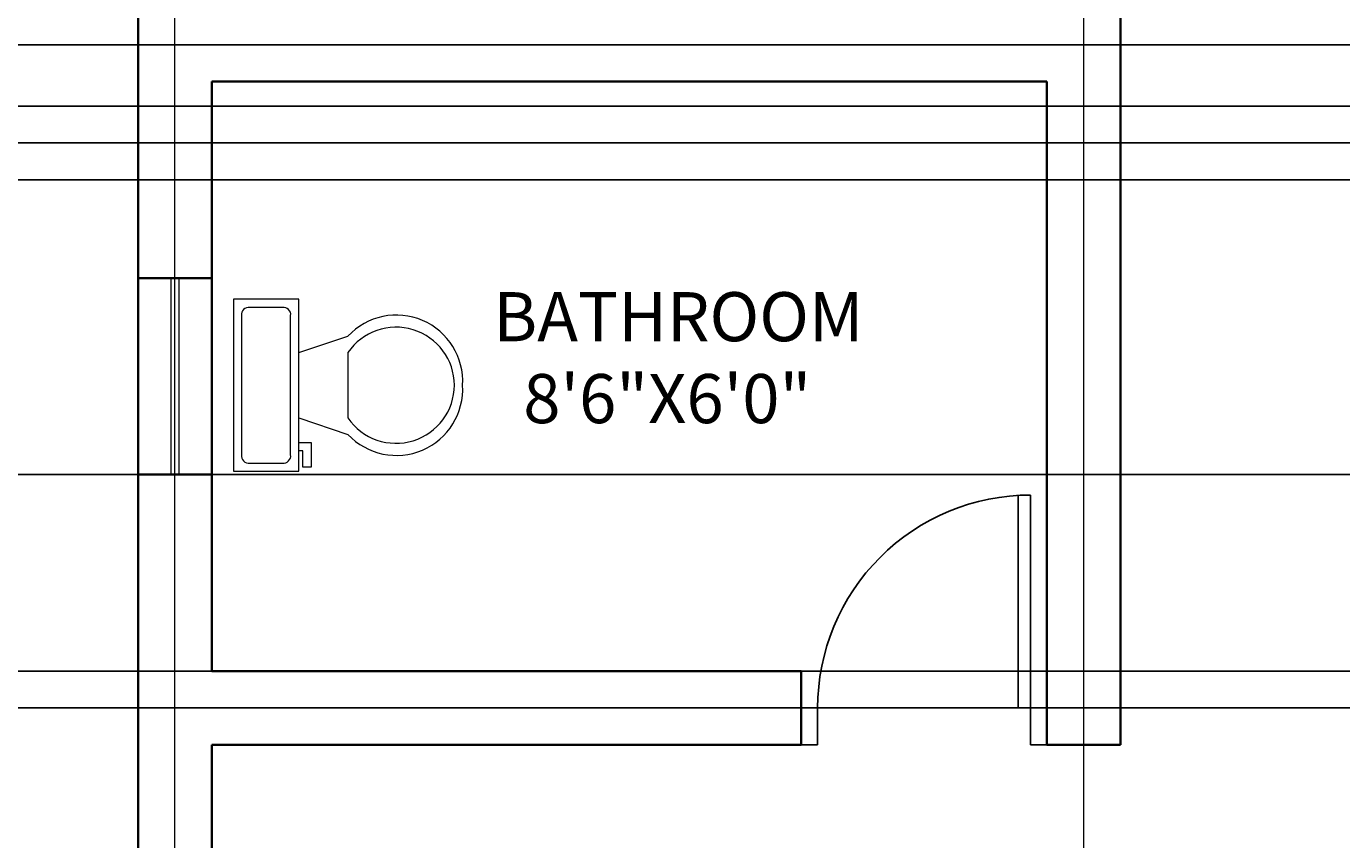
# Model space of a CAD drawing. Units: inches. Extents: x 5716 to 6907, y 12769 to 13594.
# Tile 12 of 17: x 6254 to 6414, y 13105 to 13204. Entities that reach past the tile are written whole.
import ezdxf

# ---------------------------------------------------------------- set-up
doc = ezdxf.new("R2010")
doc.units = ezdxf.units.IN
for name, color, linetype, lineweight in [('A-ANNO-DIMS', 2, 'Continuous', 18), ('A-AREA-IDEN', 7, 'Continuous', 18), ('A-DOOR', 4, 'Continuous', 25), ('A-FLOR-FIXT', 9, 'Continuous', 18), ('A-FURN', 8, 'Continuous', 18), ('A-GLAZ', 4, 'Continuous', 18), ('A-GRID', 8, 'Continuous', 13), ('A-WALL', 7, 'Continuous', 35)]:
    doc.layers.add(name, color=color, linetype=linetype, lineweight=lineweight)
doc.styles.get("Standard").update_dxf_attribs({"font": 'arial.ttf'})
doc.dimstyles.get("Standard").update_dxf_attribs({"dimtxt": 0.18, "dimasz": 0.18, "dimexe": 0.18, "dimexo": 0.0625, "dimgap": 0.09, "dimtad": 0, "dimtih": 1, "dimtoh": 1, "dimdec": 4, "dimzin": 0, "dimdsep": 46, "dimtxsty": 'Standard', "dimcen": 0.09, "dimadec": 0, "dimazin": 0, "dimtfac": 1, "dimtdec": 4, "dimtofl": 0, "dimtmove": 0, "dimatfit": 3, "dimfxl": 1, "dimtolj": 1, "dimtzin": 0, "dimarcsym": 0})

# ---------------------------------------------------------------- blocks, each defined once
blk = doc.blocks.new('A$C405465A0')
for p, q in [((1.1305, 2.1034), (1.5301, 2.1034)), ((1.5301, 2.0534), (1.1305, 2.0534)), ((1.1304, 1.6481), (1.1055, 2.0017)), ((1.279, 2.0284), (1.1105, 1.9312)), ((1.4665, 2.0284), (1.1178, 1.8271)), ((1.1305, 2.0284), (1.5301, 2.0284)), ((1.1428, 1.625), (1.1428, 2.0284)), ((1.5427, 1.8271), (1.1941, 2.0284)), ((1.2365, 1.625), (1.2365, 2.0284)), ((1.3303, 1.625), (1.3303, 2.0284)), ((1.5501, 1.9312), (1.3816, 2.0284)), ((1.424, 1.625), (1.424, 2.0284)), ((1.5178, 1.625), (1.5178, 2.0284)), ((1.555, 2.0017), (1.5301, 1.6481)), ((1.5354, 1.7231), (1.1078, 1.97)), ((1.5528, 1.97), (1.1252, 1.7231)), ((0.9452, 1.8803), (0.5455, 1.8803)), ((2.1342, 1.8803), (1.7345, 1.8803)), ((0.5455, 1.8303), (0.9452, 1.8303)), ((1.5178, 1.625), (1.1157, 1.8572)), ((1.5449, 1.8572), (1.1428, 1.625)), ((1.7345, 1.8303), (2.1342, 1.8303)), ((0.5268, 1.6904), (0.7259, 1.8053)), ((0.9452, 1.8053), (0.5455, 1.8053)), ((0.5578, 1.6), (0.5578, 1.8053)), ((0.5578, 1.6), (0.9134, 1.8053)), ((0.5773, 1.8053), (0.9328, 1.6)), ((0.6516, 1.6), (0.6516, 1.8053)), ((0.7453, 1.6), (0.7453, 1.8053)), ((0.7648, 1.8053), (0.9639, 1.6904)), ((0.8391, 1.6), (0.8391, 1.8053)), ((0.9328, 1.6), (0.9328, 1.8053)), ((1.7158, 1.6904), (1.9149, 1.8053)), ((2.1342, 1.8053), (1.7345, 1.8053)), ((1.7468, 1.6), (1.7468, 1.8053)), ((1.7468, 1.6), (2.1024, 1.8053)), ((1.7663, 1.8053), (2.1218, 1.6)), ((1.8406, 1.6), (1.8406, 1.8053)), ((1.9343, 1.6), (1.9343, 1.8053)), ((1.9538, 1.8053), (2.1529, 1.6904)), ((2.0281, 1.6), (2.0281, 1.8053)), ((2.1218, 1.6), (2.1218, 1.8053)), ((0.5206, 1.7786), (0.5332, 1.6)), ((0.9575, 1.6), (0.9701, 1.7786)), ((1.3303, 1.625), (1.1237, 1.7443)), ((1.5369, 1.7443), (1.3303, 1.625)), ((1.7096, 1.7786), (1.7222, 1.6)), ((2.1465, 1.6), (2.1591, 1.7786)), ((0.5242, 1.7277), (0.7453, 1.6)), ((0.7453, 1.6), (0.9665, 1.7277)), ((1.7132, 1.7277), (1.9343, 1.6)), ((1.9343, 1.6), (2.1555, 1.7277)), ((1.1428, 1.625), (1.1316, 1.6315)), ((1.5052, 1.625), (1.1554, 1.625)), ((1.529, 1.6315), (1.5178, 1.625)), ((2.3803, 1.6), (0.2803, 1.6)), ((0.2803, 1.6), (0.2803, 0.5)), ((0.4356, 1.5842), (0.3956, 1.553)), ((0.5827, 1.5379), (0.4356, 1.5842)), ((0.5321, 1.6149), (0.5578, 1.6)), ((0.5332, 1.6), (0.9575, 1.6)), ((0.7152, 1.6), (0.7236, 1.5766)), ((0.7236, 1.5766), (0.7578, 1.4998)), ((0.9055, 1.5469), (0.8836, 1.6)), ((0.9328, 1.6), (0.9586, 1.6149)), ((1.0212, 1.6), (1.0194, 1.5656)), ((1.1269, 1.5706), (1.1432, 1.6)), ((1.1922, 1.5507), (1.214, 1.6)), ((1.3907, 1.6), (1.3616, 1.5541)), ((1.7211, 1.6149), (1.7468, 1.6)), ((1.7222, 1.6), (2.1465, 1.6)), ((1.9093, 1.5754), (1.8386, 1.5427)), ((1.9386, 1.6), (1.9093, 1.5754)), ((2.1086, 1.5664), (2.17, 1.6)), ((2.1218, 1.6), (2.1476, 1.6149)), ((2.3803, 1.5967), (2.3153, 1.558)), ((2.3803, 0.5), (2.3803, 1.6)), ((0.3956, 1.553), (0.3856, 1.5163)), ((0.4482, 1.5094), (0.4582, 1.5336)), ((0.4582, 1.5336), (0.5016, 1.5339)), ((0.5016, 1.5339), (0.54, 1.5204)), ((0.6365, 1.5019), (0.5827, 1.5379)), ((0.9296, 1.4669), (0.9055, 1.5469)), ((1.0194, 1.5656), (1.026, 1.5003)), ((1.1178, 1.5243), (1.1269, 1.5706)), ((1.1887, 1.5196), (1.1922, 1.5507)), ((1.3616, 1.5541), (1.3027, 1.5125)), ((1.7679, 1.5301), (1.6627, 1.5271)), ((1.8386, 1.5427), (1.7679, 1.5301)), ((1.9962, 1.5248), (2.1086, 1.5664)), ((2.3153, 1.558), (2.1962, 1.4994)), ((0.3856, 1.5163), (0.4538, 1.4363)), ((0.4595, 1.4847), (0.4482, 1.5094)), ((0.54, 1.5204), (0.5786, 1.5)), ((0.5786, 1.5), (0.6151, 1.4744)), ((0.7193, 1.4377), (0.6365, 1.5019)), ((0.7578, 1.4998), (0.7752, 1.4525)), ((1.026, 1.5003), (1.0343, 1.4559)), ((1.1128, 1.4699), (1.1178, 1.5243)), ((1.2089, 1.4946), (1.1887, 1.5196)), ((1.2618, 1.4976), (1.2089, 1.4946)), ((1.3027, 1.5125), (1.2618, 1.4976)), ((1.446, 1.5079), (1.3392, 1.4609)), ((1.5543, 1.5261), (1.446, 1.5079)), ((1.6627, 1.5271), (1.5543, 1.5261)), ((1.717, 1.474), (1.8488, 1.4892)), ((1.8488, 1.4892), (1.9962, 1.5248)), ((2.1962, 1.4994), (2.0887, 1.4564)), ((2.215, 1.4381), (2.3447, 1.5068)), ((2.3447, 1.5068), (2.3803, 1.5269)), ((0.3744, 1.3943), (0.2803, 1.458)), ((0.4876, 1.4521), (0.4595, 1.4847)), ((0.5099, 1.4328), (0.4876, 1.4521)), ((0.6151, 1.4744), (0.6557, 1.4351)), ((0.7752, 1.4525), (0.7871, 1.4053)), ((0.9436, 1.385), (0.9296, 1.4669)), ((1.0343, 1.4559), (1.0488, 1.3883)), ((1.1133, 1.4295), (1.1128, 1.4699)), ((1.3392, 1.4609), (1.2655, 1.4131)), ((1.4396, 1.445), (1.5179, 1.4625)), ((1.5179, 1.4625), (1.717, 1.474)), ((2.0887, 1.4564), (1.9879, 1.4268)), ((0.4538, 1.4363), (0.5034, 1.394)), ((0.5366, 1.4137), (0.5099, 1.4328)), ((0.5694, 1.3947), (0.5366, 1.4137)), ((0.6557, 1.4351), (0.6746, 1.4025)), ((0.6746, 1.4025), (0.674, 1.3825)), ((0.7442, 1.4091), (0.7193, 1.4377)), ((0.746, 1.3555), (0.7442, 1.4091)), ((0.7871, 1.4053), (0.7898, 1.3706)), ((1.1222, 1.3821), (1.1133, 1.4295)), ((1.2655, 1.4131), (1.2034, 1.3712)), ((1.3398, 1.3841), (1.4396, 1.445)), ((1.9879, 1.4268), (1.8502, 1.4019)), ((2.1089, 1.3912), (2.215, 1.4381)), ((0.4543, 1.3479), (0.3744, 1.3943)), ((0.5034, 1.394), (0.551, 1.3648)), ((0.551, 1.3648), (0.5952, 1.3458)), ((0.597, 1.3823), (0.5694, 1.3947)), ((0.6281, 1.3731), (0.597, 1.3823)), ((0.654, 1.3714), (0.6281, 1.3731)), ((0.674, 1.3825), (0.654, 1.3714)), ((0.7898, 1.3706), (0.7722, 1.3216)), ((0.9447, 1.3133), (0.9436, 1.385)), ((1.0488, 1.3883), (1.0626, 1.2943)), ((1.1508, 1.3537), (1.1222, 1.3821)), ((1.2034, 1.3712), (1.1508, 1.3537)), ((1.2659, 1.3078), (1.3398, 1.3841)), ((1.4616, 1.3726), (1.4211, 1.3426)), ((1.5407, 1.3902), (1.4616, 1.3726)), ((1.6315, 1.3907), (1.5407, 1.3902)), ((1.7291, 1.3922), (1.6315, 1.3907)), ((1.8502, 1.4019), (1.7291, 1.3922)), ((1.8869, 1.3472), (1.9689, 1.3731)), ((1.9689, 1.3731), (2.0551, 1.3789)), ((2.0551, 1.3789), (2.1089, 1.3912)), ((2.1327, 1.3477), (2.1998, 1.3905)), ((2.1998, 1.3905), (2.271, 1.4021)), ((2.271, 1.4021), (2.3264, 1.3943)), ((2.3264, 1.3943), (2.3803, 1.3943)), ((0.2803, 1.3424), (0.3226, 1.3046)), ((0.523, 1.3203), (0.4543, 1.3479)), ((0.6007, 1.301), (0.523, 1.3203)), ((0.5952, 1.3458), (0.6524, 1.335)), ((0.6524, 1.335), (0.7159, 1.3352)), ((0.7159, 1.3352), (0.746, 1.3555)), ((0.7722, 1.3216), (0.7385, 1.3018)), ((1.4211, 1.3426), (1.398, 1.3071)), ((1.8267, 1.2783), (1.8309, 1.3257)), ((1.8309, 1.3257), (1.8869, 1.3472)), ((2.1112, 1.3052), (2.1327, 1.3477)), ((2.2336, 1.2914), (2.2346, 1.3391)), ((2.2346, 1.3391), (2.2726, 1.3593)), ((2.2726, 1.3593), (2.339, 1.3581)), ((2.339, 1.3581), (2.3803, 1.3581)), ((0.3797, 1.2052), (0.2803, 1.2816)), ((0.3226, 1.3046), (0.3891, 1.2586)), ((0.6623, 1.3018), (0.6007, 1.301)), ((0.7385, 1.3018), (0.6623, 1.3018)), ((0.9305, 1.2479), (0.9447, 1.3133)), ((1.0626, 1.2943), (1.06, 1.2384)), ((1.1689, 1.1968), (1.2659, 1.3078)), ((1.398, 1.3071), (1.412, 1.2681)), ((1.8814, 1.2462), (1.8267, 1.2783)), ((2.1264, 1.2714), (2.1112, 1.3052)), ((2.2746, 1.2504), (2.2336, 1.2914)), ((0, 1.2499), (0, 0.8502)), ((0.05, 0.8502), (0.05, 1.2499)), ((0.075, 1.0695), (0.19, 1.2686)), ((0.075, 1.2499), (0.075, 0.8502)), ((0.2803, 1.2375), (0.075, 1.2375)), ((0.075, 0.882), (0.2803, 1.2375)), ((0.2803, 1.2622), (0.1018, 1.2748)), ((0.2803, 1.05), (0.1526, 1.2712)), ((0.2803, 1.2375), (0.2654, 1.2633)), ((0.2803, 0.8379), (0.2803, 1.2622)), ((0.2803, 1.2498), (0.478, 1.1251)), ((0.3891, 1.2586), (0.4808, 1.2074)), ((0.8894, 1.1911), (0.9305, 1.2479)), ((1.06, 1.2384), (1.0402, 1.1815)), ((1.412, 1.2681), (1.4535, 1.2416)), ((1.4535, 1.2416), (1.5203, 1.2085)), ((1.9819, 1.2225), (1.8814, 1.2462)), ((2.171, 1.2386), (2.1264, 1.2714)), ((2.2593, 1.2028), (2.171, 1.2386)), ((2.3417, 1.2285), (2.2746, 1.2504)), ((2.3803, 1.2622), (2.5588, 1.2748)), ((2.3803, 1.05), (2.508, 1.2712)), ((2.3803, 1.2375), (2.3951, 1.2633)), ((2.3803, 0.8379), (2.3803, 1.2622)), ((2.3803, 1.2375), (2.5856, 1.2375)), ((2.5856, 0.882), (2.3803, 1.2375)), ((2.5856, 1.0695), (2.4706, 1.2686)), ((2.5856, 1.2499), (2.5856, 0.8502)), ((2.6106, 0.8502), (2.6106, 1.2499)), ((2.6606, 1.2499), (2.6606, 0.8502)), ((0.2803, 0.8625), (0.075, 1.2181)), ((0.3728, 1.1548), (0.2803, 1.2123)), ((0.4682, 1.1454), (0.3797, 1.2052)), ((0.4808, 1.2074), (0.5771, 1.1712)), ((0.8213, 1.159), (0.8894, 1.1911)), ((1.0809, 1.1136), (1.1689, 1.1968)), ((1.5203, 1.2085), (1.5912, 1.2143)), ((1.5912, 1.2143), (1.7027, 1.2151)), ((1.7027, 1.2151), (1.8282, 1.1987)), ((1.8282, 1.1987), (1.9236, 1.1792)), ((2.1048, 1.2108), (1.9819, 1.2225)), ((2.1888, 1.194), (2.1048, 1.2108)), ((2.2653, 1.1704), (2.1888, 1.194)), ((2.3339, 1.1841), (2.2593, 1.2028)), ((2.3803, 1.226), (2.3417, 1.2285)), ((2.3803, 0.8625), (2.5856, 1.2181)), ((0.4405, 1.1078), (0.3728, 1.1548)), ((0.5771, 1.1712), (0.7161, 1.1491)), ((0.7161, 1.1491), (0.8213, 1.159)), ((1.0402, 1.1815), (0.9932, 1.1252)), ((1.4537, 1.1662), (1.3237, 1.1316)), ((1.6097, 1.1755), (1.4537, 1.1662)), ((1.757, 1.1624), (1.6097, 1.1755)), ((1.9184, 1.131), (1.757, 1.1624)), ((1.9236, 1.1792), (2.049, 1.1552)), ((2.049, 1.1552), (2.1515, 1.1303)), ((2.3396, 1.1432), (2.2653, 1.1704)), ((2.3803, 1.1754), (2.3339, 1.1841)), ((0.2803, 1.1438), (0.075, 1.1438)), ((0.2803, 1.1471), (0.3609, 1.0879)), ((0.5402, 1.0464), (0.4405, 1.1078)), ((0.5225, 1.114), (0.4682, 1.1454)), ((0.478, 1.1251), (0.576, 1.067)), ((0.5954, 1.0801), (0.5225, 1.114)), ((0.9932, 1.1252), (0.9121, 1.0739)), ((0.9908, 1.0561), (1.0809, 1.1136)), ((1.3237, 1.1316), (1.2549, 1.1012)), ((1.4887, 1.0901), (1.6473, 1.1088)), ((1.6473, 1.1088), (1.7544, 1.0961)), ((2.0769, 1.0887), (1.9184, 1.131)), ((2.1515, 1.1303), (2.2486, 1.0908)), ((2.3803, 1.126), (2.3396, 1.1432)), ((2.3803, 1.1438), (2.5856, 1.1438)), ((0.3609, 1.0879), (0.5015, 1.0099)), ((0.576, 1.067), (0.7146, 1.0163)), ((0.6603, 1.0585), (0.5954, 1.0801)), ((0.9121, 1.0739), (0.863, 1.056)), ((1.2549, 1.1012), (1.1432, 1.0368)), ((1.3755, 1.0479), (1.4887, 1.0901)), ((1.7544, 1.0961), (1.9207, 1.0564)), ((2.2686, 1.0282), (2.0769, 1.0887)), ((2.2486, 1.0908), (2.3803, 1.048)), ((0.2803, 1.05), (0.075, 1.05)), ((0.19, 0.8315), (0.075, 1.0306)), ((0.1526, 0.8289), (0.2803, 1.05)), ((0.3078, 1.029), (0.2803, 1.0458)), ((0.346, 1.0052), (0.3078, 1.029)), ((0.6261, 1.0028), (0.5402, 1.0464)), ((0.7308, 1.0454), (0.6603, 1.0585)), ((0.7897, 1.0439), (0.7308, 1.0454)), ((0.863, 1.056), (0.7897, 1.0439)), ((0.7979, 1.0084), (0.9069, 1.0237)), ((0.9069, 1.0237), (0.9908, 1.0561)), ((1.1432, 1.0368), (1.0559, 0.9876)), ((1.2543, 0.9907), (1.3755, 1.0479)), ((1.9207, 1.0564), (2.1244, 0.9922)), ((2.3803, 0.9983), (2.2686, 1.0282)), ((2.3803, 1.05), (2.5856, 1.05)), ((2.508, 0.8289), (2.3803, 1.05)), ((2.4706, 0.8315), (2.5856, 1.0306)), ((0.4051, 0.9771), (0.346, 1.0052)), ((0.5015, 1.0099), (0.6086, 0.961)), ((0.7415, 0.9604), (0.6261, 1.0028)), ((0.7146, 1.0163), (0.7979, 1.0084)), ((1.0559, 0.9876), (0.958, 0.9508)), ((1.1244, 0.9348), (1.2543, 0.9907)), ((2.1244, 0.9922), (2.2495, 0.9522)), ((0.2803, 0.9563), (0.075, 0.9563)), ((0.4579, 0.9575), (0.4051, 0.9771)), ((0.5195, 0.9378), (0.4579, 0.9575)), ((0.5818, 0.918), (0.5195, 0.9378)), ((0.6086, 0.961), (0.7339, 0.9201)), ((0.8579, 0.9417), (0.7415, 0.9604)), ((0.958, 0.9508), (0.8579, 0.9417)), ((1.4378, 0.9282), (1.5224, 0.9439)), ((1.5224, 0.9439), (1.6187, 0.9581)), ((1.6187, 0.9581), (1.7607, 0.9676)), ((1.7607, 0.9676), (1.9339, 0.9563)), ((1.9339, 0.9563), (2.0478, 0.9301)), ((2.2495, 0.9522), (2.3803, 0.9025)), ((2.3803, 0.9563), (2.5856, 0.9563)), ((0.309, 0.9074), (0.2803, 0.9224)), ((0.342, 0.8943), (0.309, 0.9074)), ((0.3823, 0.8837), (0.342, 0.8943)), ((0.6352, 0.8954), (0.5818, 0.918)), ((0.6712, 0.8671), (0.6352, 0.8954)), ((0.7339, 0.9201), (0.8463, 0.9008)), ((0.8463, 0.9008), (0.9714, 0.9002)), ((0.9714, 0.9002), (1.1244, 0.9348)), ((1.224, 0.8829), (1.301, 0.9003)), ((1.301, 0.9003), (1.4378, 0.9282)), ((2.0478, 0.9301), (2.1209, 0.9013)), ((2.1209, 0.9013), (2.214, 0.8459)), ((0.2803, 0.8625), (0.075, 0.8625)), ((0.2654, 0.8368), (0.2803, 0.8625)), ((0.4349, 0.876), (0.3823, 0.8837)), ((0.4843, 0.8652), (0.4349, 0.876)), ((0.5229, 0.85), (0.4843, 0.8652)), ((0.6805, 0.8424), (0.6712, 0.8671)), ((0.9468, 0.8025), (1.1125, 0.8545)), ((1.1125, 0.8545), (1.224, 0.8829)), ((1.5313, 0.864), (1.3995, 0.834)), ((1.6341, 0.8806), (1.5313, 0.864)), ((1.7415, 0.8904), (1.6341, 0.8806)), ((1.8296, 0.8853), (1.7415, 0.8904)), ((1.9317, 0.8609), (1.8296, 0.8853)), ((2.0406, 0.8138), (1.9317, 0.8609)), ((2.3803, 0.8625), (2.5856, 0.8625)), ((2.3951, 0.8368), (2.3803, 0.8625)), ((0.1018, 0.8253), (0.2803, 0.8379)), ((0.5441, 0.8372), (0.5229, 0.85)), ((0.5622, 0.8164), (0.5441, 0.8372)), ((0.5634, 0.7968), (0.5622, 0.8164)), ((0.6434, 0.7666), (0.675, 0.8159)), ((0.675, 0.8159), (0.6805, 0.8424)), ((1.3995, 0.834), (1.2818, 0.7979)), ((2.1229, 0.7618), (2.0406, 0.8138)), ((2.214, 0.8459), (2.297, 0.7736)), ((2.5588, 0.8253), (2.3803, 0.8379)), ((0.5313, 0.7537), (0.5562, 0.7809)), ((0.5562, 0.7809), (0.5634, 0.7968)), ((0.603, 0.7231), (0.6434, 0.7666)), ((0.8288, 0.7556), (0.9468, 0.8025)), ((1.2818, 0.7979), (1.131, 0.7357)), ((1.4547, 0.7504), (1.6229, 0.7863)), ((1.6229, 0.7863), (1.7436, 0.7907)), ((1.7436, 0.7907), (1.8858, 0.7711)), ((1.8858, 0.7711), (1.9957, 0.7333)), ((2.297, 0.7736), (2.3432, 0.7176)), ((0.4801, 0.7185), (0.5313, 0.7537)), ((0.5568, 0.6828), (0.603, 0.7231)), ((0.6995, 0.6921), (0.8288, 0.7556)), ((1.131, 0.7357), (0.9946, 0.6604)), ((1.2995, 0.6899), (1.4547, 0.7504)), ((1.9957, 0.7333), (2.0772, 0.6873)), ((2.1698, 0.724), (2.1229, 0.7618)), ((2.2541, 0.6328), (2.1698, 0.724)), ((0.3723, 0.6742), (0.4317, 0.6944)), ((0.4317, 0.6944), (0.4801, 0.7185)), ((0.499, 0.6426), (0.5568, 0.6828)), ((0.6181, 0.6464), (0.6995, 0.6921)), ((1.2062, 0.6433), (1.2995, 0.6899)), ((1.4772, 0.6838), (1.4124, 0.6631)), ((1.554, 0.696), (1.4772, 0.6838)), ((1.6333, 0.6993), (1.554, 0.696)), ((1.7153, 0.696), (1.6333, 0.6993)), ((1.7865, 0.6892), (1.7153, 0.696)), ((1.8794, 0.6748), (1.7865, 0.6892)), ((2.0772, 0.6873), (2.1261, 0.6491)), ((2.3432, 0.7176), (2.3803, 0.6555)), ((0.2803, 0.6573), (0.312, 0.6622)), ((0.312, 0.6622), (0.3723, 0.6742)), ((0.4497, 0.615), (0.499, 0.6426)), ((0.5546, 0.6082), (0.6181, 0.6464)), ((0.9946, 0.6604), (0.8746, 0.5766)), ((1.1078, 0.5882), (1.2062, 0.6433)), ((1.4124, 0.6631), (1.3518, 0.6302)), ((1.4712, 0.6079), (1.5115, 0.6388)), ((1.5115, 0.6388), (1.5744, 0.6543)), ((1.5744, 0.6543), (1.6677, 0.668)), ((1.6031, 0.6361), (1.6918, 0.6436)), ((1.6677, 0.668), (1.7434, 0.6684)), ((1.6918, 0.6436), (1.8075, 0.6404)), ((1.7434, 0.6684), (1.8417, 0.6617)), ((1.8075, 0.6404), (1.8682, 0.6312)), ((1.8417, 0.6617), (1.8785, 0.6547)), ((1.8785, 0.6547), (1.9243, 0.6434)), ((1.9674, 0.6548), (1.8794, 0.6748)), ((1.9243, 0.6434), (1.9761, 0.6102)), ((2.0494, 0.621), (1.9674, 0.6548)), ((2.1261, 0.6491), (2.1688, 0.6067)), ((0.3813, 0.5837), (0.4497, 0.615)), ((0.4385, 0.5349), (0.5546, 0.6082)), ((1.3133, 0.5983), (1.2908, 0.5736)), ((1.3518, 0.6302), (1.3133, 0.5983)), ((1.3959, 0.5264), (1.4712, 0.6079)), ((1.4828, 0.5927), (1.5188, 0.6159)), ((1.5188, 0.6159), (1.6031, 0.6361)), ((1.5621, 0.583), (1.5815, 0.6002)), ((1.5815, 0.6002), (1.641, 0.6183)), ((1.641, 0.6183), (1.6861, 0.6235)), ((1.6861, 0.6235), (1.7353, 0.624)), ((1.7353, 0.624), (1.7765, 0.6204)), ((1.7765, 0.6204), (1.811, 0.6136)), ((1.811, 0.6136), (1.8414, 0.6025)), ((1.8414, 0.6025), (1.8603, 0.5873)), ((1.8682, 0.6312), (1.909, 0.622)), ((1.909, 0.622), (1.9497, 0.5991)), ((1.9497, 0.5991), (1.9595, 0.5705)), ((1.9761, 0.6102), (2.006, 0.5625)), ((2.1071, 0.5697), (2.0494, 0.621)), ((2.1688, 0.6067), (2.197, 0.5721)), ((2.3022, 0.5551), (2.2541, 0.6328)), ((0.2803, 0.5477), (0.3159, 0.5583)), ((0.3159, 0.5583), (0.3813, 0.5837)), ((0.8746, 0.5766), (0.8225, 0.5348)), ((1.0064, 0.5273), (1.1078, 0.5882)), ((1.2908, 0.5736), (1.2556, 0.52)), ((1.4736, 0.5658), (1.4828, 0.5927)), ((1.4775, 0.5489), (1.4736, 0.5658)), ((1.572, 0.557), (1.5621, 0.583)), ((1.5997, 0.5436), (1.572, 0.557)), ((1.8611, 0.5702), (1.8321, 0.5488)), ((1.8603, 0.5873), (1.8611, 0.5702)), ((1.9595, 0.5705), (1.9448, 0.5456)), ((2.006, 0.5625), (2.0103, 0.5395)), ((2.1338, 0.529), (2.1071, 0.5697)), ((2.197, 0.5721), (2.2242, 0.5314)), ((2.3248, 0.5), (2.3022, 0.5551)), ((0.3857, 0.5), (0.4385, 0.5349)), ((0.8225, 0.5348), (0.7878, 0.5)), ((0.9657, 0.5), (1.0064, 0.5273)), ((1.2556, 0.52), (1.2455, 0.5)), ((1.3784, 0.5), (1.3959, 0.5264)), ((1.5273, 0.534), (1.4775, 0.5489)), ((1.6327, 0.513), (1.5273, 0.534)), ((1.6329, 0.5353), (1.5997, 0.5436)), ((1.685, 0.5094), (1.6327, 0.513)), ((1.6895, 0.5294), (1.6329, 0.5353)), ((1.7388, 0.53), (1.6895, 0.5294)), ((1.7906, 0.5103), (1.7331, 0.5091)), ((1.7888, 0.5363), (1.7388, 0.53)), ((1.8321, 0.5488), (1.7888, 0.5363)), ((1.8503, 0.5169), (1.7906, 0.5103)), ((1.9108, 0.5271), (1.8503, 0.5169)), ((1.9448, 0.5456), (1.9108, 0.5271)), ((2.0103, 0.5395), (2.0069, 0.5)), ((2.1506, 0.5), (2.1338, 0.529)), ((2.2242, 0.5314), (2.2363, 0.5)), ((0.2803, 0.5), (2.3803, 0.5)), ((0.5126, 0.2463), (0.9147, 0.4784)), ((0.5205, 0.3591), (0.7272, 0.4784)), ((0.5285, 0.4719), (0.5397, 0.4784)), ((0.5397, 0.4784), (0.5397, 0.075)), ((0.5397, 0.4784), (0.9417, 0.2463)), ((0.5522, 0.4784), (0.9021, 0.4784)), ((0.6334, 0.4784), (0.6334, 0.075)), ((0.7272, 0.4784), (0.7272, 0.075)), ((0.7272, 0.4784), (0.9338, 0.3591)), ((0.8209, 0.4784), (0.8209, 0.075)), ((0.9147, 0.4784), (0.9147, 0.075)), ((0.9147, 0.4784), (0.9258, 0.4719)), ((1.1055, 0.3215), (1.1181, 0.5)), ((1.1091, 0.3724), (1.3303, 0.5)), ((1.1171, 0.4852), (1.1428, 0.5)), ((1.1181, 0.5), (1.5425, 0.5)), ((1.1428, 0.5), (1.1428, 0.2948)), ((1.1428, 0.5), (1.4984, 0.2948)), ((1.1622, 0.2948), (1.5178, 0.5)), ((1.2365, 0.5), (1.2365, 0.2948)), ((1.3303, 0.5), (1.3303, 0.2948)), ((1.3303, 0.5), (1.5515, 0.3724)), ((1.424, 0.5), (1.424, 0.2948)), ((1.5178, 0.5), (1.5178, 0.2948)), ((1.5178, 0.5), (1.5435, 0.4852)), ((1.5425, 0.5), (1.555, 0.3215)), ((1.7331, 0.5091), (1.685, 0.5094)), ((1.7096, 0.3215), (1.7222, 0.5)), ((1.7132, 0.3724), (1.9343, 0.5)), ((1.7211, 0.4852), (1.7468, 0.5)), ((1.7222, 0.5), (2.1465, 0.5)), ((1.7468, 0.5), (1.7468, 0.2948)), ((1.7468, 0.5), (2.1024, 0.2948)), ((1.7663, 0.2948), (2.1218, 0.5)), ((1.8406, 0.5), (1.8406, 0.2948)), ((1.9343, 0.5), (1.9343, 0.2948)), ((1.9343, 0.5), (2.1555, 0.3724)), ((2.0281, 0.5), (2.0281, 0.2948)), ((2.1218, 0.5), (2.1218, 0.2948)), ((2.1218, 0.5), (2.1476, 0.4852)), ((2.1465, 0.5), (2.1591, 0.3215)), ((0.5024, 0.1018), (0.5273, 0.4553)), ((0.927, 0.4553), (0.9519, 0.1018)), ((1.1118, 0.4097), (1.3109, 0.2948)), ((1.3497, 0.2948), (1.5488, 0.4097)), ((1.7158, 0.4097), (1.9149, 0.2948)), ((1.9538, 0.2948), (2.1529, 0.4097)), ((0.5046, 0.1334), (0.9323, 0.3803)), ((0.522, 0.3803), (0.9497, 0.1334)), ((0.5147, 0.2763), (0.8634, 0.075)), ((0.591, 0.075), (0.9396, 0.2763)), ((1.5301, 0.2948), (1.1305, 0.2948)), ((1.1305, 0.2698), (1.5301, 0.2698)), ((2.1342, 0.2948), (1.7345, 0.2948)), ((1.7345, 0.2698), (2.1342, 0.2698)), ((1.5301, 0.2198), (1.1305, 0.2198)), ((2.1342, 0.2198), (1.7345, 0.2198)), ((0.5074, 0.1723), (0.6759, 0.075)), ((0.7785, 0.075), (0.9469, 0.1723)), ((0.927, 0.075), (0.5273, 0.075)), ((0.5273, 0.05), (0.927, 0.05)), ((0.927, 0), (0.5273, 0))]:
    blk.add_line(p, q)
for centre, start, end in [((1.1305, 2.0784), 90, 270), ((1.5301, 2.0784), 270, 90), ((1.1305, 2.0034), 90, 184.0274), ((1.5301, 2.0034), 355.9726, 90), ((0.5455, 1.8553), 90, 270), ((0.9452, 1.8553), 270, 90), ((1.7345, 1.8553), 90, 270), ((2.1342, 1.8553), 270, 90), ((0.5455, 1.7803), 90, 184.0274), ((0.9452, 1.7803), 355.9726, 90), ((1.7345, 1.7803), 90, 184.0274), ((2.1342, 1.7803), 355.9726, 90), ((1.1554, 1.65), 184.3987, 270), ((1.5052, 1.65), 270, 355.6013), ((0.025, 1.2499), 0, 180), ((0.1, 1.2499), 85.9726, 180), ((2.5606, 1.2499), 0, 94.0274), ((2.6356, 1.2499), 0, 180), ((0.025, 0.8502), 180, 0), ((0.1, 0.8502), 180, 274.0274), ((2.5606, 0.8502), 265.9726, 0), ((2.6356, 0.8502), 180, 0), ((0.5522, 0.4534), 90, 175.6013), ((0.9021, 0.4534), 4.3987, 90), ((1.1305, 0.3198), 175.9726, 270), ((1.5301, 0.3198), 270, 4.0274), ((1.7345, 0.3198), 175.9726, 270), ((2.1342, 0.3198), 270, 4.0274), ((1.1305, 0.2448), 90, 270), ((1.5301, 0.2448), 270, 90), ((1.7345, 0.2448), 90, 270), ((2.1342, 0.2448), 270, 90), ((0.5273, 0.1), 175.9726, 270), ((0.927, 0.1), 270, 4.0274), ((0.5273, 0.025), 90, 270), ((0.927, 0.025), 270, 90)]:
    blk.add_arc(centre, 0.025, start, end)
blk = doc.blocks.new('*U11')
for p, q in [((9.5, -6), (9.5, -2)), ((-8, -8.5), (-8, -8)), ((-7, -8), (-7, -9.5)), ((-4, -8), (-6, -14)), ((4, -8), (6, -14)), ((-10, -8.5), (-8, -8.5)), ((-10, -9.5), (-10, -8.5)), ((-7, -9.5), (-10, -9.5)), ((4, -14), (-4, -14))]:
    blk.add_line(p, q)
blk.add_lwpolyline([(10.5, -8), (10.5, 0), (-10.5, 0), (-10.5, -8)], close=True)
for points in [[(8.5, -1), (-8.5, -1)], [(-9.5, -2), (-9.5, -6)], [(-8.5, -7), (8.5, -7)]]:
    blk.add_lwpolyline(points)
for centre, radius, start, end in [((-8.625, -1.875), 0.8839, 81.8699, 188.1301), ((8.625, -1.875), 0.8839, 351.8699, 98.1301), ((-8.625, -6.125), 0.8839, 171.869898, 278.1301), ((8.625, -6.125), 0.8839, 261.8699, 8.1301), ((-0.4772, -19.9188), 8.0953, 133.01722, 273.38), ((0.0374, -19.8731), 7.127, 124.50543, 269.7), ((-0.0373, -19.8731), 7.127, 270.3, 55.4946), ((0.4773, -19.9188), 8.0953, 266.62, 46.9828)]:
    blk.add_arc(centre, radius, start, end)
blk = doc.blocks.new('DOOR-SWING-30IN')
for p, q in [((0, 4.5), (-2, 4.5)), ((0, 0), (0, 4.5)), ((26, 0), (26, 4.5)), ((26, 4.5), (28, 4.5)), ((-2, 0), (0, 0)), ((0, -26), (0, 0)), ((0, 0), (1.5, 0)), ((1.5, -25.96), (1.5, 0)), ((28, 0), (26, 0))]:
    blk.add_line(p, q)
blk.add_arc((0, 0), 26, 270, 0)
blk = doc.blocks.new('WIN-GLAZING-24IN')
for p, q in [((0, 0), (0, -24)), ((1, 0), (1, -24))]:
    blk.add_line(p, q)
blk = doc.blocks.new('*D52')
at = {"layer": 'A-ANNO-DIMS', "color": 0, "lineweight": -2, "transparency": 16777216}
for p, q in [((6267.34, 13440.15), (5716.04, 13440.15)), ((5716.22, 13439.97), (5716.22, 13140.83)), ((5716.22, 12841.33), (5716.22, 13140.47)), ((6267.34, 12841.15), (5716.04, 12841.15))]:
    blk.add_line(p, q, dxfattribs=at)
at = {"layer": 'A-ANNO-DIMS', "color": 0, "transparency": 16777216}
for points in [[(5716.19, 13439.97), (5716.25, 13439.97), (5716.22, 13440.15)], [(5716.19, 12841.33), (5716.25, 12841.33), (5716.22, 12841.15)]]:
    blk.add_solid(points, dxfattribs=at)
at = {"layer": 'Defpoints', "color": 0, "transparency": 16777216}
for p in [(6267.41, 13440.15), (5716.22, 12841.15), (6267.41, 12841.15)]:
    blk.add_point(p, dxfattribs=at)
at = {"layer": 'A-ANNO-DIMS', "color": 0, "transparency": 16777216, "insert": (5716.22, 13140.65), "char_height": 0.18, "attachment_point": 5}
blk.add_mtext('\\A1;599', dxfattribs=at)
blk = doc.blocks.new('*D59')
at = {"layer": 'A-ANNO-DIMS', "color": 0, "lineweight": -2, "transparency": 16777216}
for p, q in [((6736.67, 13294.65), (5716.04, 13294.65)), ((5716.22, 13294.47), (5716.22, 13248.33)), ((5716.22, 13201.83), (5716.22, 13247.97)), ((6736.67, 13201.65), (5716.04, 13201.65))]:
    blk.add_line(p, q, dxfattribs=at)
at = {"layer": 'A-ANNO-DIMS', "color": 0, "transparency": 16777216}
for points in [[(5716.19, 13294.47), (5716.25, 13294.47), (5716.22, 13294.65)], [(5716.19, 13201.83), (5716.25, 13201.83), (5716.22, 13201.65)]]:
    blk.add_solid(points, dxfattribs=at)
at = {"layer": 'Defpoints', "color": 0, "transparency": 16777216}
for p in [(6736.73, 13294.65), (5716.22, 13201.65), (6736.73, 13201.65)]:
    blk.add_point(p, dxfattribs=at)
at = {"layer": 'A-ANNO-DIMS', "color": 0, "transparency": 16777216, "insert": (5716.22, 13248.15), "char_height": 0.18, "attachment_point": 5}
blk.add_mtext('\\A1;93', dxfattribs=at)
blk = doc.blocks.new('*D60')
at = {"layer": 'A-ANNO-DIMS', "color": 0, "lineweight": -2, "transparency": 16777216}
for p, q in [((6736.67, 13201.65), (5716.04, 13201.65)), ((5716.22, 13201.47), (5716.22, 13195.83)), ((5716.22, 13189.83), (5716.22, 13195.47)), ((6827.78, 13189.65), (5716.04, 13189.65))]:
    blk.add_line(p, q, dxfattribs=at)
at = {"layer": 'A-ANNO-DIMS', "color": 0, "transparency": 16777216}
for points in [[(5716.19, 13201.47), (5716.25, 13201.47), (5716.22, 13201.65)], [(5716.19, 13189.83), (5716.25, 13189.83), (5716.22, 13189.65)]]:
    blk.add_solid(points, dxfattribs=at)
at = {"layer": 'Defpoints', "color": 0, "transparency": 16777216}
for p in [(6736.73, 13201.65), (5716.22, 13189.65), (6827.84, 13189.65)]:
    blk.add_point(p, dxfattribs=at)
at = {"layer": 'A-ANNO-DIMS', "color": 0, "transparency": 16777216, "insert": (5716.22, 13195.65), "char_height": 0.18, "attachment_point": 5}
blk.add_mtext('\\A1;12', dxfattribs=at)
blk = doc.blocks.new('*D61')
at = {"layer": 'A-ANNO-DIMS', "color": 0, "lineweight": -2, "transparency": 16777216}
for p, q in [((6827.78, 13189.65), (5716.04, 13189.65)), ((5716.22, 13189.47), (5716.22, 13155.33)), ((5716.22, 13120.83), (5716.22, 13154.97)), ((6736.67, 13120.65), (5716.04, 13120.65))]:
    blk.add_line(p, q, dxfattribs=at)
at = {"layer": 'A-ANNO-DIMS', "color": 0, "transparency": 16777216}
for points in [[(5716.19, 13189.47), (5716.25, 13189.47), (5716.22, 13189.65)], [(5716.19, 13120.83), (5716.25, 13120.83), (5716.22, 13120.65)]]:
    blk.add_solid(points, dxfattribs=at)
at = {"layer": 'Defpoints', "color": 0, "transparency": 16777216}
for p in [(6827.84, 13189.65), (5716.22, 13120.65), (6736.73, 13120.65)]:
    blk.add_point(p, dxfattribs=at)
at = {"layer": 'A-ANNO-DIMS', "color": 0, "transparency": 16777216, "insert": (5716.22, 13155.15), "char_height": 0.18, "attachment_point": 5}
blk.add_mtext('\\A1;69', dxfattribs=at)
blk = doc.blocks.new('*D62')
at = {"layer": 'A-ANNO-DIMS', "color": 0, "lineweight": -2, "transparency": 16777216}
for p, q in [((6736.67, 13120.65), (5716.04, 13120.65)), ((5716.22, 13120.47), (5716.22, 13100.33)), ((5716.22, 13079.83), (5716.22, 13099.97)), ((6736.67, 13079.65), (5716.04, 13079.65))]:
    blk.add_line(p, q, dxfattribs=at)
at = {"layer": 'A-ANNO-DIMS', "color": 0, "transparency": 16777216}
for points in [[(5716.19, 13120.47), (5716.25, 13120.47), (5716.22, 13120.65)], [(5716.19, 13079.83), (5716.25, 13079.83), (5716.22, 13079.65)]]:
    blk.add_solid(points, dxfattribs=at)
at = {"layer": 'Defpoints', "color": 0, "transparency": 16777216}
for p in [(6736.73, 13120.65), (5716.22, 13079.65), (6736.73, 13079.65)]:
    blk.add_point(p, dxfattribs=at)
at = {"layer": 'A-ANNO-DIMS', "color": 0, "transparency": 16777216, "insert": (5716.22, 13100.15), "char_height": 0.18, "attachment_point": 5}
blk.add_mtext('\\A1;41', dxfattribs=at)
blk = doc.blocks.new('*D69')
at = {"layer": 'A-ANNO-DIMS', "color": 0, "lineweight": -2, "transparency": 16777216}
for p, q in [((5828.09, 13149.15), (6907.26, 13149.15)), ((6907.08, 13148.97), (6907.08, 13137.33)), ((6907.08, 13125.33), (6907.08, 13136.97)), ((5828.09, 13125.15), (6907.26, 13125.15))]:
    blk.add_line(p, q, dxfattribs=at)
at = {"layer": 'A-ANNO-DIMS', "color": 0, "transparency": 16777216}
for points in [[(6907.05, 13148.97), (6907.11, 13148.97), (6907.08, 13149.15)], [(6907.05, 13125.33), (6907.11, 13125.33), (6907.08, 13125.15)]]:
    blk.add_solid(points, dxfattribs=at)
at = {"layer": 'Defpoints', "color": 0, "transparency": 16777216}
for p in [(5828.02, 13149.15), (6907.08, 13149.15), (5828.02, 13125.15)]:
    blk.add_point(p, dxfattribs=at)
at = {"layer": 'A-ANNO-DIMS', "color": 0, "transparency": 16777216, "insert": (6907.08, 13137.15), "char_height": 0.18, "attachment_point": 5}
blk.add_mtext('\\A1;24', dxfattribs=at)
blk = doc.blocks.new('*D71')
at = {"layer": 'A-ANNO-DIMS', "color": 0, "lineweight": -2, "transparency": 16777216}
for p, q in [((6188.09, 13230.15), (6907.26, 13230.15)), ((6907.08, 13229.97), (6907.08, 13212.33)), ((6907.08, 13194.33), (6907.08, 13211.97)), ((6179.09, 13194.15), (6907.26, 13194.15))]:
    blk.add_line(p, q, dxfattribs=at)
at = {"layer": 'A-ANNO-DIMS', "color": 0, "transparency": 16777216}
for points in [[(6907.05, 13229.97), (6907.11, 13229.97), (6907.08, 13230.15)], [(6907.05, 13194.33), (6907.11, 13194.33), (6907.08, 13194.15)]]:
    blk.add_solid(points, dxfattribs=at)
at = {"layer": 'Defpoints', "color": 0, "transparency": 16777216}
for p in [(6188.02, 13230.15), (6907.08, 13230.15), (6179.02, 13194.15)]:
    blk.add_point(p, dxfattribs=at)
at = {"layer": 'A-ANNO-DIMS', "color": 0, "transparency": 16777216, "insert": (6907.08, 13212.15), "char_height": 0.18, "attachment_point": 5}
blk.add_mtext('\\A1;36', dxfattribs=at)
blk = doc.blocks.new('*D74')
at = {"layer": 'A-ANNO-DIMS', "color": 0, "lineweight": -2, "transparency": 16777216}
for p, q in [((6188.09, 13185.15), (6907.26, 13185.15)), ((6907.08, 13184.97), (6907.08, 13167.33)), ((6907.08, 13149.33), (6907.08, 13166.97)), ((6188.09, 13149.15), (6907.26, 13149.15))]:
    blk.add_line(p, q, dxfattribs=at)
at = {"layer": 'A-ANNO-DIMS', "color": 0, "transparency": 16777216}
for points in [[(6907.05, 13184.97), (6907.11, 13184.97), (6907.08, 13185.15)], [(6907.05, 13149.33), (6907.11, 13149.33), (6907.08, 13149.15)]]:
    blk.add_solid(points, dxfattribs=at)
at = {"layer": 'Defpoints', "color": 0, "transparency": 16777216}
for p in [(6188.02, 13185.15), (6907.08, 13185.15), (6188.02, 13149.15)]:
    blk.add_point(p, dxfattribs=at)
at = {"layer": 'A-ANNO-DIMS', "color": 0, "transparency": 16777216, "insert": (6907.08, 13167.15), "char_height": 0.18, "attachment_point": 5}
blk.add_mtext('\\A1;36', dxfattribs=at)

msp = doc.modelspace()

# ---------------------------------------------------------------- linework, layer by layer
at = {"layer": 'A-GRID'}
for p, q in [((6271.91, 12841.15), (6271.91, 13514.96)), ((6382.91, 12841.15), (6382.91, 13514.96)), ((6267.41, 13201.65), (6736.73, 13201.65)), ((6267.41, 13189.65), (6827.84, 13189.65)), ((6267.41, 13120.65), (6736.73, 13120.65))]:
    msp.add_line(p, q, dxfattribs=at)
at = {"layer": 'A-WALL'}
for p, q in [((6267.41, 13440.15), (6267.41, 12841.15)), ((6387.41, 13290.15), (6387.41, 13116.15)), ((6276.41, 13197.15), (6276.41, 13125.15)), ((6276.41, 13197.15), (6378.41, 13197.15)), ((6378.41, 13197.15), (6378.41, 13116.15)), ((6276.41, 13173.15), (6267.41, 13173.15)), ((6276.41, 13149.15), (6267.41, 13149.15)), ((6276.41, 13125.15), (6348.41, 13125.15)), ((6348.41, 13125.15), (6348.41, 13116.15)), ((6276.41, 13116.15), (6276.41, 12943.15)), ((6276.41, 13116.15), (6348.41, 13116.15)), ((6378.41, 13116.15), (6387.41, 13116.15))]:
    msp.add_line(p, q, dxfattribs=at)

# ---------------------------------------------------------------- block references
at = {"layer": 'A-DOOR', "rotation": 180}
msp.add_blockref('DOOR-SWING-30IN', (6376.41, 13120.65), dxfattribs=at)
at = {"layer": 'A-FLOR-FIXT', "rotation": 90}
msp.add_blockref('*U11', (6279.05, 13160.06), dxfattribs=at)
at = {"layer": 'A-FURN', "xscale": 37.79737452882042, "yscale": 37.79737452882042, "zscale": 37.79737452882042, "rotation": 270}
msp.add_blockref('A$C405465A0', (6413.46, 13243.2), dxfattribs=at)
at = {"layer": 'A-GLAZ'}
msp.add_blockref('WIN-GLAZING-24IN', (6271.41, 13173.15), dxfattribs=at)

# ---------------------------------------------------------------- texts
at = {"layer": 'A-AREA-IDEN', "insert": (6310.79, 13171.43), "char_height": 6, "attachment_point": 1}
msp.add_mtext_dynamic_manual_height_columns('BATHROOM\\P  8\'6"X6\'0"', width=67.4254, gutter_width=12.5, heights=[0], dxfattribs=at)

# ---------------------------------------------------------------- dimensions: what is measured, and where the dimension line sits
at = {"layer": 'A-ANNO-DIMS'}
for base, p1, p2, picture, middle in [((5716.22, 12841.15), (6267.41, 13440.15), (6267.41, 12841.15), '*D52', (5716.22, 13140.65)), ((5716.22, 13201.65), (6736.73, 13294.65), (6736.73, 13201.65), '*D59', (5716.22, 13248.15)), ((6907.08, 13230.15), (6179.02, 13194.15), (6188.02, 13230.15), '*D71', (6907.08, 13212.15)), ((5716.22, 13189.65), (6736.73, 13201.65), (6827.84, 13189.65), '*D60', (5716.22, 13195.65)), ((5716.22, 13120.65), (6827.84, 13189.65), (6736.73, 13120.65), '*D61', (5716.22, 13155.15)), ((6907.08, 13185.15), (6188.02, 13149.15), (6188.02, 13185.15), '*D74', (6907.08, 13167.15)), ((6907.08, 13149.15), (5828.02, 13125.15), (5828.02, 13149.15), '*D69', (6907.08, 13137.15)), ((5716.22, 13079.65), (6736.73, 13120.65), (6736.73, 13079.65), '*D62', (5716.22, 13100.15))]:
    dim = msp.add_linear_dim(base=base, p1=p1, p2=p2, angle=90, dimstyle='Standard', override={"dimdec": 0, "dimlfac": 1, "dimrnd": 0, "dimzin": 0, "dimdsep": 46, "dimlunit": 2}, dxfattribs=at)
    dim.commit()
    dim.dimension.update_dxf_attribs({"geometry": picture, "text_midpoint": middle})

doc.saveas('drawing.dxf')
